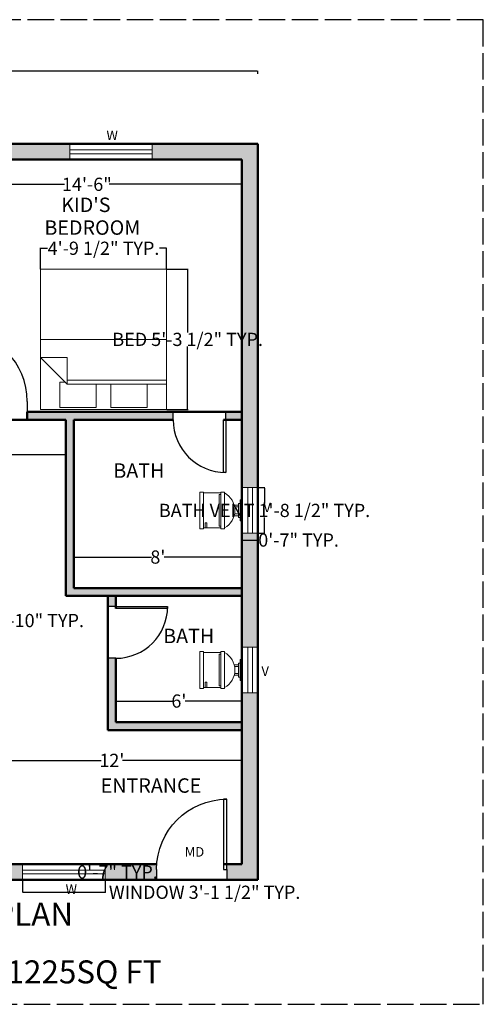
# Model space of a CAD drawing. Units: inches. Extents: x 2905 to 3459, y 4225 to 4672.
# Tile 3 of 3: x 3248 to 3459, y 4225 to 4672. Entities that reach past the tile are written whole.
import ezdxf

# ---------------------------------------------------------------- set-up
doc = ezdxf.new("R2010")
doc.units = ezdxf.units.IN
doc.header["$MEASUREMENT"] = 0
doc.linetypes.add('ACAD_ISO02W100', pattern=[15, 12, -3])
doc.layers.get('0').update_dxf_attribs({"color": 252})
for name, color, linetype, lineweight in [('A-ANNO-DIMS', 2, 'Continuous', 18), ('A-ANNO-TEXT', 7, 'Continuous', 18), ('A-ANNO-TTLB', 7, 'ACAD_ISO02W100', 25), ('A-AREA-IDEN', 7, 'Continuous', 25), ('A-DOOR', 3, 'Continuous', 25), ('A-FLOR-FIXT', 9, 'Continuous', 18), ('A-GLAZ', 4, 'Continuous', 18), ('A-WALL-PATT', 251, 'Continuous', 13), ('furniture', 8, 'Continuous', 18), ('walls', 251, 'Continuous', 50)]:
    doc.layers.add(name, color=color, linetype=linetype, lineweight=lineweight)
doc.styles.get("Standard").update_dxf_attribs({"font": 'arial.ttf'})
doc.dimstyles.get("Standard").update_dxf_attribs({"dimtxt": 6, "dimasz": 0.18, "dimexe": 0.18, "dimexo": 0.0625, "dimgap": 0.09, "dimtad": 0, "dimtih": 1, "dimtoh": 1, "dimzin": 0, "dimdsep": 46, "dimlunit": 3, "dimtxsty": 'Standard', "dimcen": 0.09, "dimadec": 0, "dimazin": 0, "dimtfac": 1, "dimtofl": 0, "dimtmove": 0, "dimatfit": 3, "dimfxl": 1, "dimtolj": 1, "dimtzin": 0, "dimarcsym": 0})

# ---------------------------------------------------------------- blocks, each defined once
blk = doc.blocks.new('*U2')
for p, q in [((0, 0), (0, -6)), ((40, 0), (40, -6))]:
    blk.add_line(p, q)
blk.add_lwpolyline([(0, 0), (0, 40), (1.75, 40), (1.75, 0)], close=True)
blk.add_arc((0, 0), 40, 0, 90)
blk = doc.blocks.new('BEDK')
at = {"layer": 'furniture'}
for p, q in [((315470.08, -113271.37), (315550.08, -113271.37)), ((315470.08, -113271.37), (315470.08, -113343.37)), ((315499.68, -113271.37), (315484.48, -113286.57)), ((315499.68, -113286.57), (315499.68, -113271.37)), ((315510.08, -113343.37), (315510.08, -113271.37)), ((315550.08, -113271.37), (315550.08, -113343.37)), ((315471.28, -113303.17), (315471.28, -113282.37)), ((315471.28, -113282.37), (315485.68, -113282.37)), ((315485.68, -113282.37), (315485.68, -113285.37)), ((315484.48, -113286.57), (315499.68, -113286.57)), ((315484.48, -113343.37), (315484.48, -113286.57)), ((315486.88, -113286.57), (315486.88, -113343.37)), ((315484.48, -113303.17), (315471.28, -113303.17)), ((315471.28, -113332.37), (315471.28, -113311.57)), ((315471.28, -113311.57), (315484.48, -113311.57)), ((315484.48, -113332.37), (315471.28, -113332.37)), ((315550.08, -113343.37), (315470.08, -113343.37))]:
    blk.add_line(p, q, dxfattribs=at)
blk = doc.blocks.new('*U4')
for p, q in [((-10, 22), (-10, 12)), ((-10, 21), (-7, 21)), ((-7, 20), (-10, 20)), ((-7, 21), (-7, 20)), ((10, 12), (10, 22)), ((10.5, 12), (-10.5, 12)), ((-10.5, 10), (-10.5, 12)), ((9, 13), (-9, 13)), ((-9, 13), (-9, 12)), ((9, 12), (9, 13)), ((10.5, 12), (10.5, 10)), ((10.5, 10), (-10.5, 10)), ((4, 2), (-4, 2)), ((-4, 2), (-4, 1)), ((-3, 4.4065), (-3, 2)), ((-2, 2), (-2, 4.1658)), ((2, 4.1658), (2, 2)), ((3, 2), (3, 4.4065)), ((4, 1), (4, 2))]:
    blk.add_line(p, q)
for points in [[(10.5, 22), (10.5, 24), (-10.5, 24), (-10.5, 22)], [(6, 0), (6, 1), (-6, 1), (-6, 0)]]:
    blk.add_lwpolyline(points, close=True)
blk.add_arc((0, 15.3333), 11.3333, 208.0725, 331.9275)
blk = doc.blocks.new('*D14')
at = {"layer": 'A-ANNO-DIMS', "color": 0, "lineweight": -2, "transparency": 16777216}
for p, q in [((3208.05, 4597.69), (3208.05, 4597.8)), ((3208.23, 4597.62), (3268.37, 4597.62)), ((3348.73, 4597.62), (3288.59, 4597.62)), ((3348.91, 4597.69), (3348.91, 4597.8))]:
    blk.add_line(p, q, dxfattribs=at)
at = {"layer": 'A-ANNO-DIMS', "color": 0, "transparency": 16777216}
for points in [[(3208.23, 4597.65), (3208.23, 4597.59), (3208.05, 4597.62)], [(3348.73, 4597.65), (3348.73, 4597.59), (3348.91, 4597.62)]]:
    blk.add_solid(points, dxfattribs=at)
at = {"layer": 'Defpoints', "color": 0, "transparency": 16777216}
for p in [(3208.05, 4597.62), (3348.91, 4597.62), (3348.91, 4597.62)]:
    blk.add_point(p, dxfattribs=at)
at = {"layer": 'A-ANNO-DIMS', "color": 0, "transparency": 16777216, "insert": (3278.48, 4597.62), "char_height": 6, "attachment_point": 5}
blk.add_mtext('\\A1;14\'-6"', dxfattribs=at)
blk = doc.blocks.new('*D15')
at = {"layer": 'A-ANNO-DIMS', "color": 0, "lineweight": -2, "transparency": 16777216}
for p, q in [((3272.51, 4428.41), (3272.51, 4428.53)), ((3272.69, 4428.35), (3307.86, 4428.35)), ((3348.73, 4428.35), (3313.57, 4428.35)), ((3348.91, 4428.41), (3348.91, 4428.53))]:
    blk.add_line(p, q, dxfattribs=at)
at = {"layer": 'A-ANNO-DIMS', "color": 0, "transparency": 16777216}
for points in [[(3272.69, 4428.38), (3272.69, 4428.32), (3272.51, 4428.35)], [(3348.73, 4428.38), (3348.73, 4428.32), (3348.91, 4428.35)]]:
    blk.add_solid(points, dxfattribs=at)
at = {"layer": 'Defpoints', "color": 0, "transparency": 16777216}
for p in [(3272.51, 4428.35), (3348.91, 4428.35), (3348.91, 4428.35)]:
    blk.add_point(p, dxfattribs=at)
at = {"layer": 'A-ANNO-DIMS', "color": 0, "transparency": 16777216, "insert": (3310.71, 4428.35), "char_height": 6, "attachment_point": 5}
blk.add_mtext("\\A1;8'", dxfattribs=at)
blk = doc.blocks.new('*D16')
at = {"layer": 'A-ANNO-DIMS', "color": 0, "lineweight": -2, "transparency": 16777216}
for p, q in [((3291.61, 4363.02), (3291.61, 4363.14)), ((3291.79, 4362.96), (3317.39, 4362.96)), ((3348.73, 4362.96), (3323.13, 4362.96)), ((3348.91, 4363.02), (3348.91, 4363.14))]:
    blk.add_line(p, q, dxfattribs=at)
at = {"layer": 'A-ANNO-DIMS', "color": 0, "transparency": 16777216}
for points in [[(3291.79, 4362.99), (3291.79, 4362.93), (3291.61, 4362.96)], [(3348.73, 4362.99), (3348.73, 4362.93), (3348.91, 4362.96)]]:
    blk.add_solid(points, dxfattribs=at)
at = {"layer": 'Defpoints', "color": 0, "transparency": 16777216}
for p in [(3291.61, 4362.96), (3348.91, 4362.96), (3348.91, 4362.96)]:
    blk.add_point(p, dxfattribs=at)
at = {"layer": 'A-ANNO-DIMS', "color": 0, "transparency": 16777216, "insert": (3320.26, 4362.96), "char_height": 6, "attachment_point": 5}
blk.add_mtext("\\A1;6'", dxfattribs=at)
blk = doc.blocks.new('*D18')
at = {"layer": 'A-ANNO-DIMS', "color": 0, "lineweight": -2, "transparency": 16777216}
for p, q in [((3230.73, 4336.07), (3230.73, 4336.19)), ((3230.91, 4336.01), (3284.92, 4336.01)), ((3348.73, 4336.01), (3294.72, 4336.01)), ((3348.91, 4336.07), (3348.91, 4336.19))]:
    blk.add_line(p, q, dxfattribs=at)
at = {"layer": 'A-ANNO-DIMS', "color": 0, "transparency": 16777216}
for points in [[(3230.91, 4336.04), (3230.91, 4335.98), (3230.73, 4336.01)], [(3348.73, 4336.04), (3348.73, 4335.98), (3348.91, 4336.01)]]:
    blk.add_solid(points, dxfattribs=at)
at = {"layer": 'Defpoints', "color": 0, "transparency": 16777216}
for p in [(3230.73, 4336.01), (3348.91, 4336.01), (3348.91, 4336.01)]:
    blk.add_point(p, dxfattribs=at)
at = {"layer": 'A-ANNO-DIMS', "color": 0, "transparency": 16777216, "insert": (3289.82, 4336.01), "char_height": 6, "attachment_point": 5}
blk.add_mtext("\\A1;12'", dxfattribs=at)
blk = doc.blocks.new('*D23')
at = {"layer": 'A-ANNO-DIMS', "color": 0, "lineweight": -2, "transparency": 16777216}
for p, q in [((3138.38, 4474.67), (3138.38, 4474.55)), ((3138.56, 4474.73), (3193.54, 4474.73)), ((3268.75, 4474.73), (3213.77, 4474.73)), ((3268.93, 4474.79), (3268.93, 4474.91))]:
    blk.add_line(p, q, dxfattribs=at)
at = {"layer": 'A-ANNO-DIMS', "color": 0, "transparency": 16777216}
for points in [[(3138.56, 4474.76), (3138.56, 4474.7), (3138.38, 4474.73)], [(3268.75, 4474.76), (3268.75, 4474.7), (3268.93, 4474.73)]]:
    blk.add_solid(points, dxfattribs=at)
at = {"layer": 'Defpoints', "color": 0, "transparency": 16777216}
for p in [(3138.38, 4474.73), (3268.93, 4474.73), (3268.93, 4474.73)]:
    blk.add_point(p, dxfattribs=at)
at = {"layer": 'A-ANNO-DIMS', "color": 0, "transparency": 16777216, "insert": (3203.66, 4474.73), "char_height": 6, "attachment_point": 5}
blk.add_mtext('\\A1;13\'-8"', dxfattribs=at)
blk = doc.blocks.new('*D26')
at = {"layer": 'A-ANNO-DIMS', "color": 0, "lineweight": -2, "transparency": 16777216}
for p, q in [((3021.82, 4647.77), (3021.82, 4649.13)), ((3022, 4648.95), (3183.77, 4648.95)), ((3355.89, 4648.95), (3194.13, 4648.95)), ((3356.07, 4647.77), (3356.07, 4649.13))]:
    blk.add_line(p, q, dxfattribs=at)
at = {"layer": 'A-ANNO-DIMS', "color": 0, "transparency": 16777216}
for points in [[(3022, 4648.98), (3022, 4648.92), (3021.82, 4648.95)], [(3355.89, 4648.98), (3355.89, 4648.92), (3356.07, 4648.95)]]:
    blk.add_solid(points, dxfattribs=at)
at = {"layer": 'Defpoints', "color": 0, "transparency": 16777216}
for p in [(3021.82, 4647.71), (3356.07, 4648.95), (3356.07, 4647.71)]:
    blk.add_point(p, dxfattribs=at)
at = {"layer": 'A-ANNO-DIMS', "color": 0, "transparency": 16777216, "insert": (3188.95, 4648.95), "char_height": 6, "attachment_point": 5}
blk.add_mtext("\\A1;35'", dxfattribs=at)
blk = doc.blocks.new('WIN-PLAN-STANDARD')
for p, q in [((0, 7.16), (0, 0)), ((37.45, 7.16), (0, 7.16)), ((0, 7.16), (0, 4.38)), ((37.45, 0), (37.45, 7.16)), ((0, 4.38), (37.45, 4.38)), ((0, 2.7), (37.45, 2.7)), ((37.45, 4.38), (37.45, 2.7)), ((0, 0), (37.45, 0))]:
    blk.add_line(p, q)
blk = doc.blocks.new('WIN-BATH-VENT')
for p, q in [((0, 20.69), (7.16, 20.69)), ((0, 0), (0, 20.69)), ((2.65, 20.69), (2.65, 0)), ((4.77, 0), (4.77, 20.69)), ((7.16, 20.69), (7.16, 0)), ((7.16, 0), (0, 0)), ((2.65, 0), (4.77, 0))]:
    blk.add_line(p, q)
blk = doc.blocks.new('*D30')
at = {"layer": 'A-ANNO-DIMS', "color": 0, "lineweight": -2, "transparency": 16777216}
for p, q in [((3249.3, 4281.67), (3249.3, 4275.94)), ((3286.75, 4281.67), (3286.75, 4275.94)), ((3249.48, 4276.12), (3286.57, 4276.12)), ((3286.75, 4276.12), (3286.93, 4276.12))]:
    blk.add_line(p, q, dxfattribs=at)
at = {"layer": 'A-ANNO-DIMS', "color": 0, "transparency": 16777216}
for points in [[(3249.48, 4276.15), (3249.48, 4276.09), (3249.3, 4276.12)], [(3286.57, 4276.15), (3286.57, 4276.09), (3286.75, 4276.12)]]:
    blk.add_solid(points, dxfattribs=at)
at = {"layer": 'Defpoints', "color": 0, "transparency": 16777216}
for p in [(3249.3, 4281.74), (3286.75, 4281.74), (3286.75, 4276.12)]:
    blk.add_point(p, dxfattribs=at)
at = {"layer": 'A-ANNO-DIMS', "color": 0, "transparency": 16777216, "insert": (3331.97, 4276.12), "char_height": 6, "attachment_point": 5}
blk.add_mtext('\\A1;WINDOW 3\'-1 1/2" TYP.', dxfattribs=at)
blk = doc.blocks.new('*D31')
at = {"layer": 'A-ANNO-DIMS', "color": 0, "lineweight": -2, "transparency": 16777216}
for p, q in [((3286.81, 4288.9), (3292.55, 4288.9)), ((3292.37, 4288.72), (3292.37, 4288.47)), ((3286.81, 4281.74), (3292.55, 4281.74)), ((3292.37, 4281.92), (3292.37, 4282.16))]:
    blk.add_line(p, q, dxfattribs=at)
at = {"layer": 'A-ANNO-DIMS', "color": 0, "transparency": 16777216}
for points in [[(3292.34, 4288.72), (3292.4, 4288.72), (3292.37, 4288.9)], [(3292.34, 4281.92), (3292.4, 4281.92), (3292.37, 4281.74)]]:
    blk.add_solid(points, dxfattribs=at)
at = {"layer": 'Defpoints', "color": 0, "transparency": 16777216}
for p in [(3286.75, 4288.9), (3292.37, 4288.9), (3286.75, 4281.74)]:
    blk.add_point(p, dxfattribs=at)
at = {"layer": 'A-ANNO-DIMS', "color": 0, "transparency": 16777216, "insert": (3292.37, 4285.32), "char_height": 6, "attachment_point": 5}
blk.add_mtext('\\A1;0\'-7" TYP.', dxfattribs=at)
blk = doc.blocks.new('*D32')
at = {"layer": 'A-ANNO-DIMS', "color": 0, "lineweight": -2, "transparency": 16777216}
for p, q in [((3168.67, 4396.25), (3168.67, 4399.69)), ((3168.85, 4399.51), (3190.61, 4399.51)), ((3190.79, 4396.25), (3190.79, 4399.69)), ((3190.79, 4399.51), (3190.97, 4399.51))]:
    blk.add_line(p, q, dxfattribs=at)
at = {"layer": 'A-ANNO-DIMS', "color": 0, "transparency": 16777216}
for points in [[(3168.85, 4399.54), (3168.85, 4399.48), (3168.67, 4399.51)], [(3190.61, 4399.54), (3190.61, 4399.48), (3190.79, 4399.51)]]:
    blk.add_solid(points, dxfattribs=at)
at = {"layer": 'Defpoints', "color": 0, "transparency": 16777216}
for p in [(3168.67, 4396.19), (3190.79, 4399.51), (3190.79, 4396.19)]:
    blk.add_point(p, dxfattribs=at)
at = {"layer": 'A-ANNO-DIMS', "color": 0, "transparency": 16777216, "insert": (3235.37, 4399.51), "char_height": 6, "attachment_point": 5}
blk.add_mtext('\\A1;ARMCHAIR 1\'-10" TYP.', dxfattribs=at)
blk = doc.blocks.new('*D34')
at = {"layer": 'A-ANNO-DIMS', "color": 0, "lineweight": -2, "transparency": 16777216}
for p, q in [((3314.75, 4559.03), (3324.42, 4559.03)), ((3324.24, 4558.85), (3324.24, 4530.39)), ((3324.24, 4495.54), (3324.24, 4524)), ((3314.75, 4495.36), (3324.42, 4495.36))]:
    blk.add_line(p, q, dxfattribs=at)
at = {"layer": 'A-ANNO-DIMS', "color": 0, "transparency": 16777216}
for points in [[(3324.21, 4558.85), (3324.27, 4558.85), (3324.24, 4559.03)], [(3324.21, 4495.54), (3324.27, 4495.54), (3324.24, 4495.36)]]:
    blk.add_solid(points, dxfattribs=at)
at = {"layer": 'Defpoints', "color": 0, "transparency": 16777216}
for p in [(3314.69, 4559.03), (3324.24, 4559.03), (3314.69, 4495.36)]:
    blk.add_point(p, dxfattribs=at)
at = {"layer": 'A-ANNO-DIMS', "color": 0, "transparency": 16777216, "insert": (3324.24, 4527.2), "char_height": 6, "attachment_point": 5}
blk.add_mtext('\\A1;BED 5\'-3 1/2" TYP.', dxfattribs=at)
blk = doc.blocks.new('*D35')
at = {"layer": 'A-ANNO-DIMS', "color": 0, "lineweight": -2, "transparency": 16777216}
for p, q in [((3257.39, 4559.09), (3257.39, 4568.76)), ((3257.57, 4568.58), (3260.55, 4568.58)), ((3314.51, 4568.58), (3311.53, 4568.58)), ((3314.69, 4559.09), (3314.69, 4568.76))]:
    blk.add_line(p, q, dxfattribs=at)
at = {"layer": 'A-ANNO-DIMS', "color": 0, "transparency": 16777216}
for points in [[(3257.57, 4568.61), (3257.57, 4568.55), (3257.39, 4568.58)], [(3314.51, 4568.61), (3314.51, 4568.55), (3314.69, 4568.58)]]:
    blk.add_solid(points, dxfattribs=at)
at = {"layer": 'Defpoints', "color": 0, "transparency": 16777216}
for p in [(3257.39, 4568.58), (3257.39, 4559.03), (3314.69, 4559.03)]:
    blk.add_point(p, dxfattribs=at)
at = {"layer": 'A-ANNO-DIMS', "color": 0, "transparency": 16777216, "insert": (3286.04, 4568.58), "char_height": 6, "attachment_point": 5}
blk.add_mtext('\\A1;4\'-9 1/2" TYP.', dxfattribs=at)
blk = doc.blocks.new('*D36')
at = {"layer": 'A-ANNO-DIMS', "color": 0, "lineweight": -2, "transparency": 16777216}
for p, q in [((3356.14, 4459.86), (3359.36, 4459.86)), ((3359.18, 4459.68), (3359.18, 4452.71)), ((3359.18, 4439.35), (3359.18, 4446.32)), ((3356.14, 4439.17), (3359.36, 4439.17))]:
    blk.add_line(p, q, dxfattribs=at)
at = {"layer": 'A-ANNO-DIMS', "color": 0, "transparency": 16777216}
for points in [[(3359.15, 4459.68), (3359.21, 4459.68), (3359.18, 4459.86)], [(3359.15, 4439.35), (3359.21, 4439.35), (3359.18, 4439.17)]]:
    blk.add_solid(points, dxfattribs=at)
at = {"layer": 'Defpoints', "color": 0, "transparency": 16777216}
for p in [(3356.07, 4459.86), (3359.18, 4459.86), (3356.07, 4439.17)]:
    blk.add_point(p, dxfattribs=at)
at = {"layer": 'A-ANNO-DIMS', "color": 0, "transparency": 16777216, "insert": (3359.18, 4449.52), "char_height": 6, "attachment_point": 5}
blk.add_mtext('\\A1;BATH VENT 1\'-8 1/2" TYP.', dxfattribs=at)
blk = doc.blocks.new('*D37')
at = {"layer": 'A-ANNO-DIMS', "color": 0, "lineweight": -2, "transparency": 16777216}
for p, q in [((3348.91, 4439.11), (3348.91, 4435.89)), ((3349.09, 4436.07), (3355.89, 4436.07)), ((3356.07, 4439.11), (3356.07, 4435.89)), ((3356.07, 4436.07), (3356.25, 4436.07))]:
    blk.add_line(p, q, dxfattribs=at)
at = {"layer": 'A-ANNO-DIMS', "color": 0, "transparency": 16777216}
for points in [[(3349.09, 4436.1), (3349.09, 4436.04), (3348.91, 4436.07)], [(3355.89, 4436.1), (3355.89, 4436.04), (3356.07, 4436.07)]]:
    blk.add_solid(points, dxfattribs=at)
at = {"layer": 'Defpoints', "color": 0, "transparency": 16777216}
for p in [(3348.91, 4439.17), (3356.07, 4439.17), (3356.07, 4436.07)]:
    blk.add_point(p, dxfattribs=at)
at = {"layer": 'A-ANNO-DIMS', "color": 0, "transparency": 16777216, "insert": (3374.63, 4436.07), "char_height": 6, "attachment_point": 5}
blk.add_mtext('\\A1;0\'-7" TYP.', dxfattribs=at)

msp = doc.modelspace()

# ---------------------------------------------------------------- hatches: boundary and pattern name
at = {"layer": 'A-WALL-PATT'}
h = msp.add_hatch(color=256, dxfattribs=at)
h.dxf.hatch_style = 1
h.paths.add_polyline_path([(3291.611, 4382.367), (3288.03, 4382.367), (3288.03, 4349.781), (3348.911, 4349.781), (3348.911, 4353.362), (3291.611, 4353.362)])
h.paths.add_polyline_path([(3291.611, 4410.662), (3288.03, 4410.662), (3288.03, 4405.956), (3291.611, 4405.956)])
h.paths.add_polyline_path([(3356.074, 4439.171), (3348.911, 4439.171), (3348.911, 4387.379), (3356.074, 4387.379)])
h.paths.add_polyline_path([(3356.074, 4366.687), (3348.911, 4366.687), (3348.911, 4288.899), (3341.991, 4288.899), (3341.991, 4286.512), (3341.991, 4281.737), (3356.074, 4281.737)])
h.paths.add_polyline_path([(3310.157, 4286.512, -0.0187698), (3310.247, 4288.899), (3286.75, 4288.899), (3286.75, 4281.737), (3310.157, 4281.737)])
h.paths.add_polyline_path([(3249.298, 4288.899), (3230.73, 4288.899), (3230.73, 4346.199), (3227.148, 4346.199), (3227.148, 4288.899), (3221.363, 4288.899), (3221.363, 4281.737), (3249.298, 4281.737)])
h.paths.add_polyline_path([(3230.73, 4349.781), (3227.148, 4349.781), (3227.148, 4346.199), (3230.73, 4346.199)])
h.paths.add_polyline_path([(3183.911, 4288.899), (3169.848, 4288.899), (3169.848, 4346.199), (3166.267, 4346.199), (3166.267, 4288.899), (3158.463, 4288.899), (3158.463, 4281.737), (3183.911, 4281.737)])
h.paths.add_polyline_path([(3169.848, 4349.781), (3166.267, 4349.781), (3166.267, 4346.199), (3169.848, 4346.199)])
h.paths.add_polyline_path([(3166.267, 4349.781), (3154.383, 4349.781), (3154.383, 4346.199), (3166.267, 4346.199)])
h.paths.add_polyline_path([(3130.507, 4349.781), (3105.385, 4349.781), (3105.385, 4288.899), (3082.76, 4288.899), (3082.76, 4281.737), (3121.011, 4281.737), (3121.011, 4288.899), (3108.967, 4288.899), (3108.967, 4346.199), (3130.507, 4346.199)])
h.paths.add_polyline_path([(3045.307, 4288.899), (3028.985, 4288.899), (3028.985, 4351.673), (3021.822, 4351.673), (3021.822, 4281.737), (3045.307, 4281.737)])
h.paths.add_polyline_path([(3028.985, 4428.302), (3021.822, 4428.302), (3021.822, 4389.126), (3028.985, 4389.126), (3028.985, 4410.662), (3138.383, 4410.662), (3138.383, 4414.244), (3028.985, 4414.244)])
h.paths.add_polyline_path([(3356.074, 4615.988), (3308.212, 4615.988), (3308.212, 4608.826), (3348.911, 4608.826), (3348.911, 4459.863), (3356.074, 4459.863)])
h.paths.add_polyline_path([(3053.98, 4501.489), (3061.351, 4501.489), (3061.351, 4511.329), (3053.98, 4511.329)], flags=9)
h.paths.add_polyline_path([(3141.419, 4592.43), (3152.5, 4592.43), (3152.5, 4602.27), (3141.419, 4602.27)], flags=9)
h.paths.add_polyline_path([(3089.982, 4547.099), (3101.063, 4547.099), (3101.063, 4556.939), (3089.982, 4556.939)], flags=9)
h.paths.add_polyline_path([(3268.583, 4592.669), (3287.963, 4592.669), (3287.963, 4602.509), (3268.583, 4602.509)], flags=9)
h.paths.add_polyline_path([(3307.047, 4423.398), (3314.418, 4423.398), (3314.418, 4433.237), (3307.047, 4433.237)], flags=9)
h.paths.add_polyline_path([(3288.865, 4462.697), (3316.591, 4462.697), (3316.591, 4472.539), (3288.865, 4472.539)], flags=9)
h.paths.add_polyline_path([(3037.676, 4519.097), (3065.402, 4519.097), (3065.402, 4528.939), (3037.676, 4528.939)], flags=9)
h.paths.add_polyline_path([(3265.13, 4583.219), (3291.666, 4583.219), (3291.666, 4593.397), (3265.13, 4593.397)], flags=9)
h.paths.add_polyline_path([(3257.487, 4572.872), (3308.243, 4572.872), (3308.243, 4583.057), (3257.487, 4583.057)], flags=9)
h.paths.add_polyline_path([(3132.382, 4572.872), (3183.138, 4572.872), (3183.138, 4583.057), (3132.382, 4583.057)], flags=9)
h.paths.add_polyline_path([(3134.197, 4582.452), (3175.785, 4582.452), (3175.785, 4592.629), (3134.197, 4592.629)], flags=9)
h = msp.add_hatch(color=256, dxfattribs=at)
h.dxf.hatch_style = 1
h.paths.add_polyline_path([(3208.048, 4608.826), (3270.759, 4608.826), (3270.759, 4615.988), (3168.781, 4615.988), (3168.781, 4608.826), (3204.467, 4608.826), (3204.467, 4494.225), (3191.238, 4494.225), (3191.238, 4490.644), (3219.587, 4490.644), (3219.587, 4494.225), (3208.048, 4494.225)])
h.paths.add_polyline_path([(3089.866, 4579.625), (3086.285, 4579.625), (3086.285, 4494.225), (3028.985, 4494.225), (3028.985, 4547.094), (3021.822, 4547.094), (3021.822, 4465.755), (3028.985, 4465.755), (3028.985, 4490.644), (3159.404, 4490.644), (3159.404, 4494.225), (3089.866, 4494.225)])
h.paths.add_polyline_path([(3131.329, 4615.988), (3021.822, 4615.988), (3021.822, 4567.786), (3024.467, 4567.786), (3028.985, 4567.786), (3028.985, 4608.826), (3086.285, 4608.826), (3086.285, 4603.214), (3086.328, 4603.214), (3089.866, 4603.214), (3089.866, 4608.826), (3131.329, 4608.826)])
h = msp.add_hatch(color=256, dxfattribs=at)
h.dxf.hatch_style = 1
h.paths.add_polyline_path([(3317.701, 4494.225), (3251.421, 4494.225), (3251.421, 4490.644), (3268.93, 4490.644), (3268.93, 4410.662), (3348.911, 4410.662), (3348.911, 4414.244), (3272.511, 4414.244), (3272.511, 4490.644), (3317.701, 4490.644)])
h.paths.add_polyline_path([(3348.911, 4494.225), (3341.576, 4494.225), (3341.576, 4490.644), (3348.911, 4490.644)], flags=17)

# ---------------------------------------------------------------- linework, layer by layer
at = {"layer": 'A-ANNO-TTLB'}
for p, q in [((3458.552, 4672.373), (2904.821, 4672.373)), ((3458.552, 4225.241), (3458.552, 4672.373)), ((2904.821, 4225.241), (3458.552, 4225.241))]:
    msp.add_line(p, q, dxfattribs=at)
at = {"layer": 'walls'}
for p, q in [((3021.822, 4615.988), (3356.074, 4615.988)), ((3356.074, 4615.988), (3356.074, 4281.737)), ((3208.048, 4608.826), (3348.911, 4608.826)), ((3348.911, 4608.826), (3348.911, 4288.899)), ((3251.421, 4494.225), (3348.911, 4494.225)), ((3251.421, 4494.225), (3251.421, 4490.644)), ((3028.985, 4490.644), (3268.93, 4490.644)), ((3268.93, 4490.644), (3268.93, 4410.662)), ((3272.511, 4490.644), (3272.511, 4414.244)), ((3272.511, 4490.644), (3317.701, 4490.644)), ((3340.532, 4490.644), (3348.911, 4490.644)), ((3272.511, 4414.244), (3348.911, 4414.244)), ((3268.93, 4410.662), (3348.911, 4410.662)), ((3288.03, 4410.662), (3288.03, 4349.781)), ((3291.611, 4410.662), (3291.611, 4404.924)), ((3291.611, 4382.367), (3291.611, 4353.362)), ((3288.03, 4353.362), (3288.03, 4349.781)), ((3291.611, 4353.362), (3348.911, 4353.362)), ((3288.03, 4349.781), (3348.911, 4349.781)), ((3348.911, 4349.781), (3288.03, 4349.781)), ((3310.247, 4288.899), (3230.73, 4288.899)), ((3348.911, 4288.899), (3340.598, 4288.899)), ((3356.074, 4281.737), (3021.822, 4281.737))]:
    msp.add_line(p, q, dxfattribs=at)

# ---------------------------------------------------------------- block references
at = {"layer": 'A-DOOR', "yscale": 0.7958373047019981, "zscale": 0.7958373047019981}
for p, xscale in [((3219.587, 4499), 0.7958373047019981), ((3341.991, 4286.512), -0.7958373047019981)]:
    msp.add_blockref('*U2', p, dxfattribs=dict(at, xscale=xscale))
at = {"layer": 'A-DOOR'}
for p, xscale, yscale, zscale, rotation in [((3341.576, 4490.644), 0.5968803451172152, 0.5968803451172152, 0.5968803451172152, 180), ((3291.568, 4405.956), 0.58972064018156, 0.58972064018156, 0.58972064018156, 270)]:
    msp.add_blockref('*U2', p, dxfattribs=dict(at, xscale=xscale, yscale=yscale, zscale=zscale, rotation=rotation))
at = {"layer": 'A-FLOR-FIXT', "xscale": 0.7958373047019981, "yscale": 0.7958373047019981, "zscale": 0.7958373047019981, "rotation": 90}
for p in [(3348.911, 4449.517), (3348.911, 4377.033)]:
    msp.add_blockref('*U4', p, dxfattribs=at)
at = {"layer": 'A-GLAZ'}
for name, p in [('WIN-PLAN-STANDARD', (3270.759, 4608.826)), ('WIN-BATH-VENT', (3348.911, 4439.171)), ('WIN-BATH-VENT', (3348.911, 4366.687)), ('WIN-PLAN-STANDARD', (3249.297, 4281.737))]:
    msp.add_blockref(name, p, dxfattribs=at)
at = {"layer": 'furniture', "xscale": 0.7958373047019981, "yscale": 0.7958373047019981, "zscale": 0.7958373047019981, "rotation": 89.99999999999996}
msp.add_blockref('BEDK', (-86888.191, -246567.499), dxfattribs=at)

# ---------------------------------------------------------------- texts
at = {"layer": 'A-ANNO-TEXT'}
for s, height, p in [('W', 4.319, (3287.378, 4617.687)), ('V', 4.319, (3358.649, 4448.749)), ('V', 4.319, (3357.77, 4374.392)), ('MD', 4.3194, (3322.936, 4292.295)), ('W', 4.319, (3268.819, 4275.374)), ('GROUND FLOOR PLAN', 10.45739, (3124.308, 4260.929)), ('TOTAL BUILDUP AREA=1225SQ FT', 10.45739, (3088.083, 4234.734))]:
    msp.add_text(s, height=height, dxfattribs=at).set_placement(p)
at = {"layer": 'A-AREA-IDEN'}
for s, p in [("KID'S", (3266.826, 4585.027)), ('BEDROOM', (3259.184, 4574.682)), ('BATH', (3290.505, 4464.337)), ('BATH', (3313.138, 4389.246)), ('ENTRANCE', (3284.747, 4321.305))]:
    msp.add_text(s, height=6.5613, dxfattribs=at).set_placement(p)

# ---------------------------------------------------------------- dimensions: what is measured, and where the dimension line sits
at = {"layer": 'A-ANNO-DIMS'}
for base, p1, p2, text, override, picture, middle in [((3356.074, 4648.949), (3021.822, 4647.711), (3356.074, 4647.711), "35'", {"dimclrd": 0, "dimclre": 0, "dimclrt": 0}, '*D26', (3188.948, 4648.949)), ((3348.911, 4597.623), (3208.048, 4597.623), (3348.911, 4597.623), '14\'-6"', {"dimclrd": 0, "dimclre": 0, "dimclrt": 0}, '*D14', (3278.48, 4597.623)), ((3268.93, 4474.73), (3138.383, 4474.73), (3268.93, 4474.73), '13\'-8"', {"dimclrd": 0, "dimclre": 0, "dimclrt": 0}, '*D23', (3203.657, 4474.73)), ((3356.074, 4436.067), (3348.911, 4439.171), (3356.074, 4439.171), '<> TYP.', {"dimdec": 1, "dimlfac": 1, "dimrnd": 0, "dimzin": 1, "dimdsep": 46, "dimlunit": 4, "dimfrac": 2}, '*D37', (3374.63, 4436.067)), ((3348.911, 4428.352), (3272.511, 4428.352), (3348.911, 4428.352), "8'", {"dimclrd": 0, "dimclre": 0, "dimclrt": 0}, '*D15', (3310.711, 4428.352)), ((3190.79, 4399.51), (3168.667, 4396.191), (3190.79, 4396.191), 'ARMCHAIR <> TYP.', {"dimdec": 1, "dimlfac": 1, "dimrnd": 0, "dimzin": 1, "dimdsep": 46, "dimlunit": 4, "dimfrac": 2}, '*D32', (3235.368, 4399.51)), ((3348.911, 4362.955), (3291.611, 4362.955), (3348.911, 4362.955), "6'", {"dimclrd": 0, "dimclre": 0, "dimclrt": 0}, '*D16', (3320.261, 4362.955)), ((3348.911, 4336.01), (3230.73, 4336.01), (3348.911, 4336.01), "12'", {"dimclrd": 0, "dimclre": 0, "dimclrt": 0}, '*D18', (3289.821, 4336.01)), ((3286.75, 4276.119), (3249.298, 4281.737), (3286.75, 4281.737), 'WINDOW <> TYP.', {"dimdec": 1, "dimlfac": 1, "dimrnd": 0, "dimzin": 1, "dimdsep": 46, "dimlunit": 4, "dimfrac": 2}, '*D30', (3331.973, 4276.119))]:
    dim = msp.add_linear_dim(base=base, p1=p1, p2=p2, text=text, dimstyle='Standard', override=override, dxfattribs=at)
    dim.commit()
    dim.dimension.update_dxf_attribs({"geometry": picture, "text_midpoint": middle})
for base, p1, p2, angle, text, picture, middle in [((3257.39, 4568.579), (3314.69, 4559.029), (3257.39, 4559.029), 180, '<> TYP.', '*D35', (3286.04, 4568.579)), ((3324.24, 4559.029), (3314.69, 4495.362), (3314.69, 4559.029), 90, 'BED <> TYP.', '*D34', (3324.24, 4527.196)), ((3359.178, 4459.863), (3356.074, 4439.171), (3356.074, 4459.863), 90, 'BATH VENT <> TYP.', '*D36', (3359.178, 4449.517)), ((3292.368, 4288.899), (3286.75, 4281.737), (3286.75, 4288.899), 90, '<> TYP.', '*D31', (3292.368, 4285.318))]:
    dim = msp.add_linear_dim(base=base, p1=p1, p2=p2, angle=angle, text=text, dimstyle='Standard', override={"dimdec": 1, "dimlfac": 1, "dimrnd": 0, "dimzin": 1, "dimdsep": 46, "dimlunit": 4, "dimfrac": 2}, dxfattribs=at)
    dim.commit()
    dim.dimension.update_dxf_attribs({"geometry": picture, "text_midpoint": middle})

doc.saveas('drawing.dxf')
